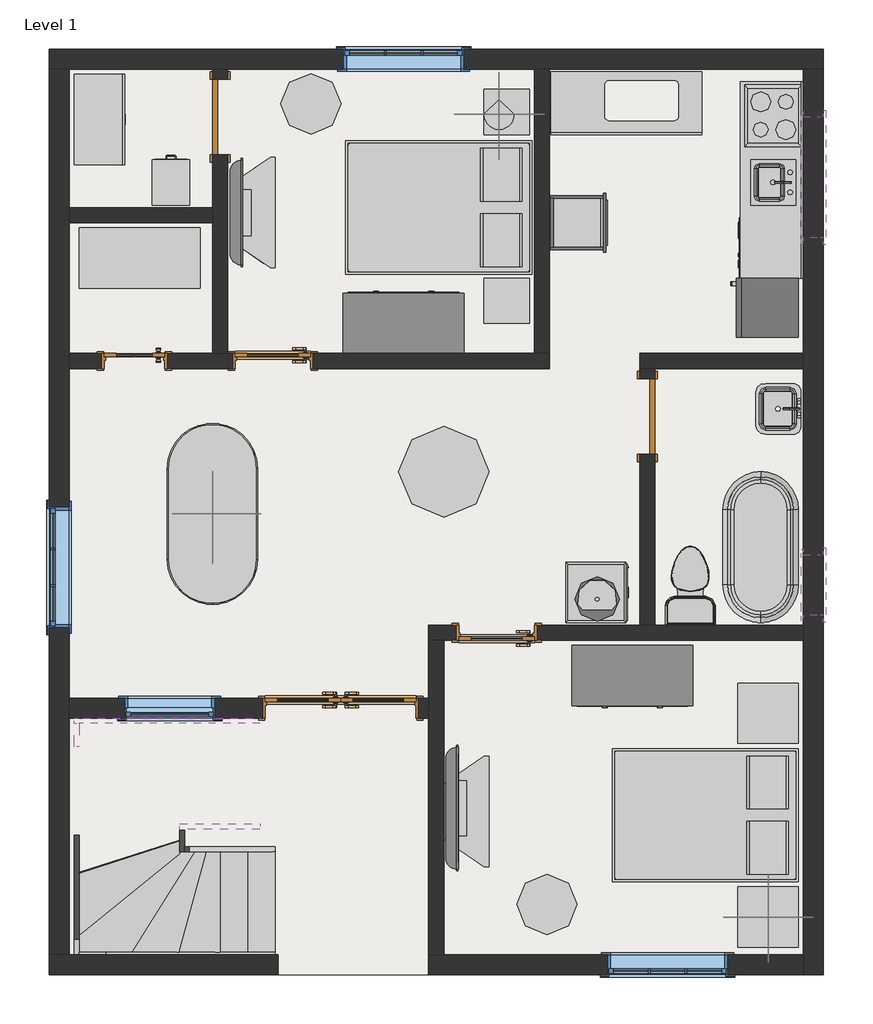
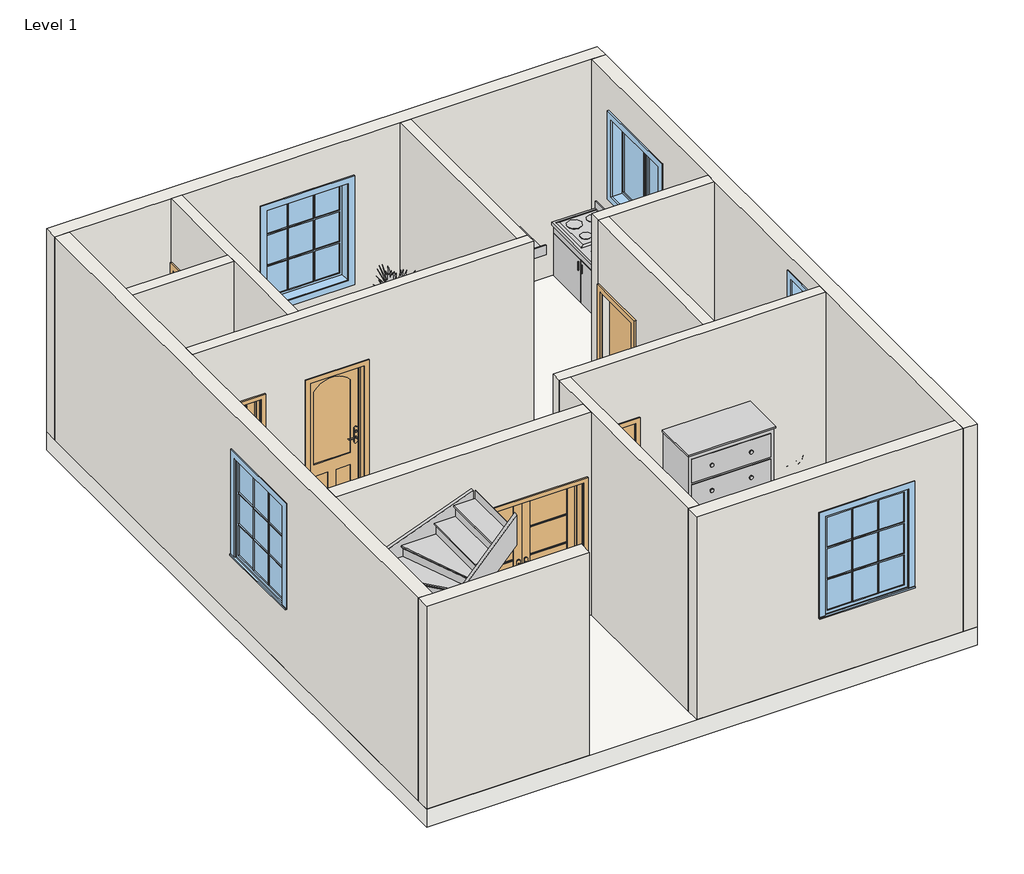
# One storey, incomplete: 22 furniture elements, 14 walls, 8 members, 6 doors, 6 windows, 5 flow terminals, 5 proxies, 3 geographic elements, 2 other elements.
# Revit data of these elements (continued)
# Type "Casement 3x3 with Trim : 48\" x 60\"" (continued)
#   Define Thermal Properties by = 1
#   Glass Pane Material = Glass
#   Sash Material = Sash
#   Trim Exterior Material = Trim
#   Trim Interior Material = Trim
#   Wall Closure = (empty or 0)
# Type "Casement Dbl with Trim : 48\" x 48\""
#   Type Mark = "13"
#   Construction Type Id = "GSP4R"
#   Assembly Code = "B2020100"
#   Analytic Construction = "1/8 in Pilkington single glazing"
#   Visual Light Transmittance = 0.9
#   Solar Heat Gain Coefficient = 0.78
#   Heat Transfer Coefficient (U) = 0.6496 BTU/(h·ft²·°F)
#   Height = 4' - 0"
#   Default Sill Height = 3' - 0"
#   Trim Projection - Ext. = 0' - 0 1/2"
#   Trim Projection - Int. = 0' - 0 3/4"
#   Trim Width - Exterior = 0' - 3 1/2"
#   Trim Width - Interior = 0' - 3 1/2"
#   Width = 4' - 0"
#   Window Inset = 0' - 0 3/4"
#   Define Thermal Properties by = 1
#   Glass Pane Material = Glass
#   Sash Material = Sash
#   Trim Exterior Material = Trim
#   Trim Interior Material = Trim
#   Wall Closure = (empty or 0)
# Type "Double Hung with Trim : 36\" x 48\""
#   Type Mark = "16"
#   Construction Type Id = "GSP4R"
#   Assembly Code = "B2020100"
#   Analytic Construction = "1/8 in Pilkington single glazing"
#   Visual Light Transmittance = 0.9
#   Solar Heat Gain Coefficient = 0.78
#   Heat Transfer Coefficient (U) = 0.6496 BTU/(h·ft²·°F)
#   Height = 4' - 0"
#   Default Sill Height = 3' - 0"
#   Trim Projection - Ext. = 0' - 0 1/2"
#   Trim Projection - Int. = 0' - 0 3/4"
#   Trim Width - Exterior = 0' - 3 1/2"
#   Trim Width - Interior = 0' - 3 1/2"
#   Width = 3' - 0"
#   Window Inset = 0' - 0 3/4"
#   Define Thermal Properties by = 1
#   Glass Pane Material = Glass
#   Sash Material = Sash
#   Trim Exterior Material = Trim
#   Trim Interior Material = Trim
#   Wall Closure = (empty or 0)
# Type "Transom with Trim : 24\" x 24\""
#   Type Mark = "25"
#   Construction Type Id = "GSP4R"
#   Assembly Code = "B2020100"
#   Analytic Construction = "1/8 in Pilkington single glazing"
#   Visual Light Transmittance = 0.9
#   Solar Heat Gain Coefficient = 0.78
#   Heat Transfer Coefficient (U) = 0.6496 BTU/(h·ft²·°F)
#   Height = 2' - 0"
#   Default Sill Height = 7' - 1"
#   Trim Projection - Ext. = 0' - 0 1/2"
#   Trim Projection - Int. = 0' - 0 3/4"
#   Trim Width - Exterior = 0' - 3 1/2"
#   Trim Width - Interior = 0' - 3 1/2"
#   Width = 2' - 0"
#   Window Inset = 0' - 0 3/4"
#   Define Thermal Properties by = 1
#   Glass Pane Material = Glass
#   Sash Material = Sash
#   Trim Exterior Material = Trim
#   Trim Interior Material = Trim
#   Wall Closure = (empty or 0)
# Element 1 (IfcBuildingElementProxy, "Cook Top-4 Unit2 : 22\" x 20\"")
#   Phase Created = New Construction
#   Materials on its faces: "Steel, Chrome Plated", "Steel, Polished"
# Element 2 (IfcBuildingElementProxy, "Dishwasher : 24\" x 24\" x 34\"")
#   Phase Created = New Construction
#   Materials on its faces: "Steel, Paint Finish, Ivory, Glossy", "Plastic, Opaque Black"
# Element 3 (IfcBuildingElementProxy, "Kitchenette - Medium : Kitchenette - Medium")
#   Phase Created = New Construction
#   Materials on its faces: "Cabinets", "Cabinets - Handles"
# Element 4 (IfcBuildingElementProxy, "Oven Double-Built-in : 21 1/2\" x 39 1/4\" x 21\"")
#   Phase Created = New Construction
#   Materials on its faces: "Steel", "Metal - Stainless Steel, Polished", "Glass"
# Element 5 (IfcBuildingElementProxy, "Refrigerator : 24\" x 25\" LH")
#   Phase Created = New Construction
#   Materials on its faces: "Steel, Paint Finish, Ivory, Glossy", "Steel, Chrome Plated"
# Elements 6, 7 (IfcDoor, "30\" x 80\"")
#   Threshold Offset = 0' - 0 1/2"
#   Swing Angle = 90.00°
#   Door Offset = 0' - 0"
#   Threshold = yes
#   Exterior Trim = yes
#   Phase Created = New Construction
#   Materials on its faces: "Cherry", "Aluminum", "Glass"
# Element 8 (IfcDoor, "Door-Exterior-Double-Full Glass-Wood_Clad : 60\" x 80\"")
#   Threshold Offset = 0' - 0 1/2"
#   Swing Angle = 90.00°
#   Door Offset = 0' - 0"
#   Threshold = yes
#   Show Grill = yes
#   Exterior Trim = yes
#   Phase Created = New Construction
#   Materials on its faces: "Cherry", "Aluminum", "Glass"
# Element 9 (IfcDoor, "Door-Interior-Single-Full Glass-Wood : 24\" x 80\"")
#   Swing Angle = 90.00°
#   Show Grill = yes
#   Phase Created = New Construction
#   Materials on its faces: "Cherry", "Aluminum", "Glass"
# Elements 10, 11 (IfcDoor, "Single-Flush : 30\" x 80\"")
#   Phase Created = New Construction
#   Materials on its faces: "Door - Frame", "Door - Panel"
# Element 12 (IfcFlowTerminal, "Sink Kitchen-Island : 18\" x 18\"")
#   Mark = "5"
#   Phase Created = New Construction
#   Materials on its faces: "Steel, Polished"
# Element 13 (IfcFlowTerminal, "Sink Vanity-Round : 19\" x 19\"")
#   Mark = "6"
#   Phase Created = New Construction
#   Materials on its faces: "Porcelain, Linen", "Steel, Polished"
# Element 14 (IfcFlowTerminal, "Sink Vanity-Square : 20\" x 18\"")
#   Mark = "4"
#   Phase Created = New Construction
#   Materials on its faces: "Porcelain, Linen", "Steel, Polished"
# Element 15 (IfcFlowTerminal, "Toilet-Domestic-3D : Toilet-Domestic-3D")
#   Mark = "1"
#   Phase Created = New Construction
#   Materials on its faces: "Porcelain, Linen", "Laminate, Linen, Matte"
# Element 16 (IfcFlowTerminal, "Tub-Free Standing-3D : 30\" x 60\"")
#   Mark = "2"
#   Phase Created = New Construction
#   Materials on its faces: "Porcelain, Ivory"
# Element 17 (IfcFurniture, "24\"")
#   Phase Created = New Construction
#   Materials on its faces: "Cabinets", "Cabinets - Handles"
# Elements 18, 19 (IfcFurniture, "Bed-Box : Double 53\" x 74\"")
#   Phase Created = New Construction
#   Materials on its faces: "Birch", "Linen, White"
# Element 20 (IfcFurniture, "Cabinet-File 3 Drawer.0001 : 15\" x 18\"")
#   Phase Created = New Construction
#   Materials on its faces: "Steel, Chrome Plated", "Steel, Paint Finish, Ivory, Glossy"
# Element 21 (IfcFurniture, "Counter Top w Sink Hole : 24\" Depth")
#   Sink Opening Depth = 1' - 2"
#   Sink Location To Wall = 0' - 6"
#   Length = 6' - 6"
#   Sink Location = 3' - 4"
#   Sink Opening Width = 1' - 4"
#   Phase Created = New Construction
#   Materials on its faces: "Counter Top"
# Element 22 (IfcFurniture, "Counter Top w Sink Hole : 24\" Depth")
#   Sink Opening Width = 2' - 4.37215"
#   Sink Opening Depth = 1' - 3"
#   Sink Location To Wall = 0' - 6"
#   Sink Location = 2' - 0"
#   Length = 5' - 0"
#   Phase Created = New Construction
#   Materials on its faces: "Counter Top"
# Element 23 (IfcFurniture, "Dresser : 48\" x 60\" x 24\"")
#   Phase Created = New Construction
#   Materials on its faces: "Laminate, Ivory, Matte", "Cherry", "Laminate - Ivory, Glossy"
# Element 24 (IfcFurniture, "Dresser : 48\" x 72\" x 24\"")
#   Phase Created = New Construction
#   Materials on its faces: "Laminate, Ivory, Matte", "Cherry", "Laminate - Ivory, Glossy"
# Element 25 (IfcFurniture, "Storage Pedestal : 20\" x 36\" x 36\"")
#   Phase Created = New Construction
#   Materials on its faces: "Steel, Paint Finish, Ivory, Glossy", "Steel, Chrome Plated"
# Element 26 (IfcFurniture, "TV - Flat Screen : 42\"")
#   Stand = yes
#   Phase Created = New Construction
#   Materials on its faces: "TV - Black", "TV - Glass", "TV - Screen"
# Element 27 (IfcFurniture, "TV - Flat Screen : 50\"")
#   Stand = yes
#   Phase Created = New Construction
#   Materials on its faces: "TV - Black", "TV - Glass", "TV - Screen"
# Elements 28, 29 (IfcFurniture, "TV Stand : TV Stand")
#   Phase Created = New Construction
#   Materials on its faces: "Melamine - Gray", "Glass - Shelves"
# Element 30 (IfcFurniture, "Table-Dining Oval : 36\" x 72\"")
#   Phase Created = New Construction
#   Materials on its faces: "Steel, Chrome Plated", "Glass - Clear, Grey"
# Element 31 (IfcFurniture, "Table-Dining Round w Chairs : 36\" Diameter")
#   Phase Created = New Construction
#   Materials on its faces: "Pine", "Laminate, Linen, Matte"
# Elements 32, 33 (IfcFurniture, "Table-Ellipse : 72\" x 36\"")
#   Phase Created = New Construction
#   Materials on its faces: "Birch", "Laminate - Black"
# Elements 34, 35 (IfcFurniture, "Table-Night Stand : 18\" x 18\" x 24\"")
#   Phase Created = New Construction
#   Materials on its faces: "Birch", "Laminate, Ivory, Matte"
# Elements 36, 37 (IfcFurniture, "Table-Night Stand : 24\" x 24\" x 30\"")
#   Phase Created = New Construction
#   Materials on its faces: "Birch", "Laminate, Ivory, Matte"
# Element 38 (IfcFurniture, "Table-Rectangular : 72\" x 30\"")
#   Phase Created = New Construction
#   Materials on its faces: "Birch"
# Element 39 (IfcGeographicElement, "RPC Plant - Tropical")
#   Phase Created = New Construction
# Elements 40, 41 (IfcGeographicElement, "RPC Plant - Tropical : Agave - 1.5'")
#   Phase Created = New Construction
# Elements 42, 43, 44, 45, 46, 47, 48, 49 (IfcMember, "Stringer - 2\" Width")
#   Phase Created = New Construction
# Element 50 (IfcSlab, "Wood Joist 10\" - Ceramic Tile")
#   Height Offset From Level = 0' - 0"
#   Phase Created = New Construction
#   Materials on its faces: "Structure, Wood Joist/Rafter Layer", "Tile, Mosaic, Gray"
# Element 51 (IfcStairFlight, "2\" Tread 1\" Nosing 1/4\" Riser")
#   Phase Created = New Construction
# Elements 52, 53, 54, 55, 56, 57 (IfcWall, "Generic - 8\"")
#   Top Offset = 0' - 0"
#   Base Offset = 0' - 0"
#   Unconnected Height = 10' - 0"
#   wall height = 10' - 0"
#   Phase Created = New Construction
#   Base Constraint = Level 1
#   Materials on its faces: "Brick, Common"
# Elements 58, 59, 60, 61, 62, 63, 64, 65 (IfcWall, "INNER WALL")
#   Top Offset = 0' - 0"
#   Base Offset = 0' - 0"
#   Unconnected Height = 10' - 0"
#   wall height = 10' - 0"
#   Phase Created = New Construction
#   Base Constraint = Level 1
#   Materials on its faces: "Brick, Common"
# Element 66 (IfcWindow, "Casement 3x3 with Trim : 48\" x 60\"")
#   Mark = "1"
#   Phase Created = New Construction
#   Materials on its faces: "Sash", "Glass", "Trim"
# Element 67 (IfcWindow, "Casement 3x3 with Trim : 48\" x 60\"")
#   Mark = "2"
#   Phase Created = New Construction
#   Materials on its faces: "Sash", "Glass", "Trim"
# Element 68 (IfcWindow, "Casement 3x3 with Trim : 48\" x 60\"")
#   Mark = "3"
#   Phase Created = New Construction
#   Materials on its faces: "Sash", "Glass", "Trim"
# Element 69 (IfcWindow, "Casement Dbl with Trim : 48\" x 48\"")
#   Mark = "4"
#   Phase Created = New Construction
#   Materials on its faces: "Sash", "Trim", "Glass"
# Element 70 (IfcWindow, "Double Hung with Trim : 36\" x 48\"")
#   Mark = "6"
#   Phase Created = New Construction
#   Materials on its faces: "Sash", "Trim", "Glass"
# Element 71 (IfcWindow, "Transom with Trim : 24\" x 24\"")
#   Mark = "7"
#   Phase Created = New Construction
#   Materials on its faces: "Sash", "Trim", "Glass"
# Materials
#   "Steel, Chrome Plated": class "Metal", colour RGB 17 17 17, transparency 0, Description = "Chromiuim plated steel", Cost = 0
#   "Steel, Polished": class "Metal", colour RGB 57 57 57, transparency 0, Description = "Polished steel", Cost = 0
#   "Steel, Paint Finish, Ivory, Glossy": class "Metal", colour RGB 247 247 239, transparency 0, Description = "Steel, paint finish, ivory, glossy", Cost = 0
#   "Plastic, Opaque Black": class "Plastic", colour RGB 0 0 0, transparency 0.7, Description = "Plastic, generic, opaque black", Cost = 0
#   "Cabinets": colour RGB 249 249 249, transparency 0
#   "Cabinets - Handles": class "Metal", colour RGB 57 57 57, transparency 0
#   "Metal - Stainless Steel, Polished": class "Metal", colour RGB 216 216 216, transparency 0
#   "Cherry": class "Wood", colour RGB 226 177 128, transparency 0, Description = "Prunus Serotina", Cost = 0
#   "Glass": class "Glass", colour RGB 0 128 192, transparency 0.75, Description = "Soda Lime Glass", Cost = 0
#   "Aluminum": class "Metal", colour RGB 247 247 247, transparency 0, Description = "Aluminum 6061", Cost = 0
#   "Door - Panel": class "Wood", colour RGB 210 159 95, transparency 0
#   "Door - Frame": colour RGB 118 70 51, transparency 0
#   "Porcelain, Linen": class "Ceramic", colour RGB 249 239 230, transparency 0, Description = "Porcelain, linen", Cost = 0
#   "Laminate, Linen, Matte": class "Plastic", colour RGB 249 239 230, transparency 0, Description = "Plastic Laminate - Linen, Matte", Cost = 0
#   "Porcelain, Ivory": class "Ceramic", colour RGB 247 247 239, transparency 0, Description = "Porcelain, ivory", Cost = 0
#   "Birch": class "Wood", colour RGB 224 178 126, transparency 0, Description = "Betula Alleghaniensis", Cost = 0
#   "Linen, White": class "Textile", colour RGB 247 247 239, transparency 0, Description = "Linen, white", Cost = 0
#   "Laminate - Ivory, Glossy": colour RGB 247 247 239, transparency 0
#   "Laminate, Ivory, Matte": class "Plastic", colour RGB 247 247 239, transparency 0, Description = "Plastic Laminate - Ivory, Matte", Cost = 0
#   "Melamine - Gray": class "Wood", colour RGB 49 49 49, transparency 0
#   "Glass - Clear, Grey": class "Glass", colour RGB 252 255 255, transparency 0.64
#   "Pine": class "Wood", colour RGB 223 192 134, transparency 0, Description = "Pinus Echinata", Cost = 0
#   "Laminate - Black": colour RGB 0 0 0, transparency 0
#   "Tile, Mosaic, Gray": class "Generic", colour RGB 127 127 127, transparency 0, Description = "Mosiac tile, gray", Cost = 0
#   "Concrete, Cast-in-Place gray": class "Concrete", colour RGB 192 192 192, transparency 0, Description = "Cast-in-place concrete", Cost = 0
#   "Plywood, Sheathing": class "Wood", colour RGB 212 179 113, transparency 0, Description = "Plywood, sheathing grade", Cost = 0
#   "Structure, Wood Joist/Rafter Layer": class "Wood", colour RGB 127 127 127, transparency 0, Description = "Wood framing, thermal airspace", Cost = 0
#   "Brick, Common": class "Masonry", colour RGB 170 98 104, transparency 0, Description = "Common brick", Cost = 0
#   "Sash": class "Wood", colour RGB 224 178 126, transparency 0
#   "Trim": class "Wood", colour RGB 224 178 126, transparency 0
#   "Steel": class "Metal", colour RGB 247 247 247, transparency 0, Description = "Steel, mill finish", Cost = 0
#   "Counter Top": class "Wood", colour RGB 226 177 128, transparency 0
#   "TV - Black": colour RGB 49 49 49, transparency 0
#   "TV - Glass": colour RGB 157 157 157, transparency 0.9
#   "TV - Screen": colour RGB 0 0 0, transparency 0
#   "Glass - Shelves": class "Glass", colour RGB 167 167 167, transparency 0.9
# Room at (-7292.493, 5497.572) mm, phase "New Construction", upper level "Level 1", upper offset 10' - 0", lower offset 0' - 0"
#   Number = "1"
#   Name = "PORCH"
# Room at (-4214.355, 6005.306) mm, phase "New Construction", upper level "Level 1", upper offset 10' - 0", lower offset 0' - 0"
#   Number = "2"
#   Name = "BED ROOM"
# Room at (-3348.086, 8702.644) mm, phase "New Construction", upper level "Level 1", upper offset 10' - 0", lower offset 0' - 0"
#   Number = "3"
#   Name = "TOILET"
# Room at (-6308.758, 9384.911) mm, phase "New Construction", upper level "Level 1", upper offset 10' - 0", lower offset 0' - 0"
#   Number = "4"
#   Name = "DRAWING HALL"
# Room at (-3817.687, 12066.382) mm, phase "New Construction", upper level "Level 1", upper offset 10' - 0", lower offset 0' - 0"
#   Number = "5"
#   Name = "KITCHEN"
# Room at (-6737.159, 12066.382) mm, phase "New Construction", upper level "Level 1", upper offset 10' - 0", lower offset 0' - 0"
#   Number = "6"
#   Name = "BED ROOM"
# Room at (-9019.693, 12494.783) mm, phase "New Construction", upper level "Level 1", upper offset 10' - 0", lower offset 0' - 0"
#   Number = "7"
#   Name = "STORE"
# Room at (-9355.163, 11232.628) mm, phase "New Construction", upper level "Level 1", upper offset 10' - 0", lower offset 0' - 0"
#   Number = "8"
